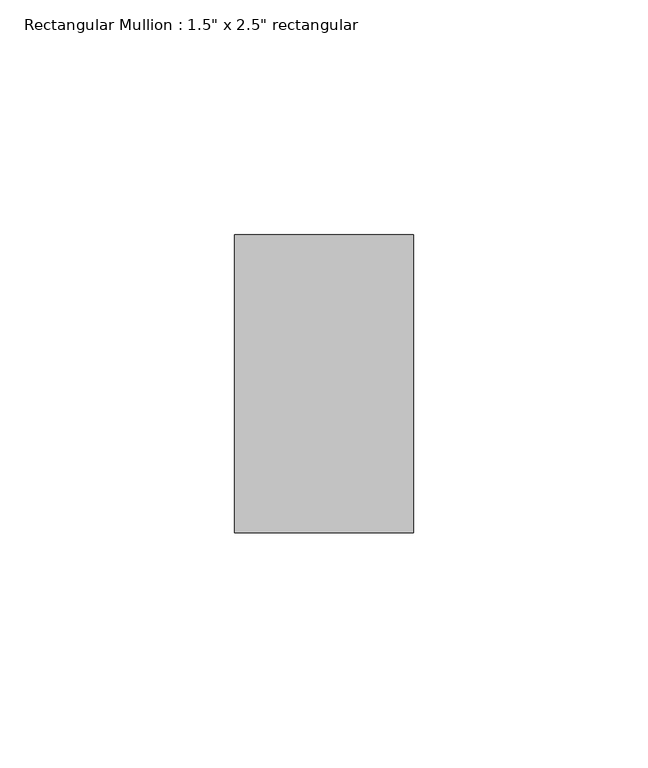
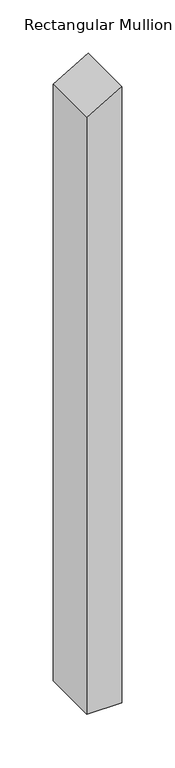
"""IFC4 building model written with IfcOpenShell, lengths in millimetres: member geometry."""

from ifc_helpers import new_model, si_unit, frame, origin, place, context, project, spatial, polyline, outline, extrude, source, transform, mapped, element, save


def member_83e1ecc3(model_context):
    return source(origin(), model_context, "Body", "SweptSolid", [
        extrude(outline(polyline([(0.0, 0.0), (-22.6445139, -38.1), (-709.1419508, -38.1), (-709.1419508, 0.0), (0.0, 0.0)])), frame((0.0, -31.75, 0.0), z_axis=(0.0, 1.0, 0.0), x_axis=(0.0, 0.0, 1.0)), (0.0, 0.0, 1.0), 63.5),
    ])


if __name__ == "__main__":
    model = new_model("IFC4")
    model_context = context("Model", 3, world=origin())
    ifc_project = project(units=[si_unit("LENGTHUNIT", "METRE", prefix="MILLI")], contexts=[model_context])
    site = spatial("IfcSite", under=ifc_project)
    building = spatial("IfcBuilding", under=site)
    placement = place(None, origin())
    member_shape = member_83e1ecc3(model_context)
    element("IfcMember", 1, ObjectType="Rectangular Mullion : 1.5\" x 2.5\" rectangular", at=placement, inside=building, context=model_context, shape_type="MappedRepresentation", body=[
        mapped(member_shape, transform((0.0, 0.0, 0.0), x_axis=(1.0, 0.0, 0.0), y_axis=(0.0, 1.0, 0.0), z_axis=(0.0, 0.0, 1.0))),
    ])
    save(model, "model.ifc")

# Revit data of these elements
# Type "Rectangular Mullion : 1.5\" x 2.5\" rectangular"
#   built-in parameter 1007304 = 0.208333 (stored number, unit not read)
#   built-in parameter 1007301 = 0.0625 (stored number, unit not read)
#   built-in parameter 1007300 = 0.0625 (stored number, unit not read)
